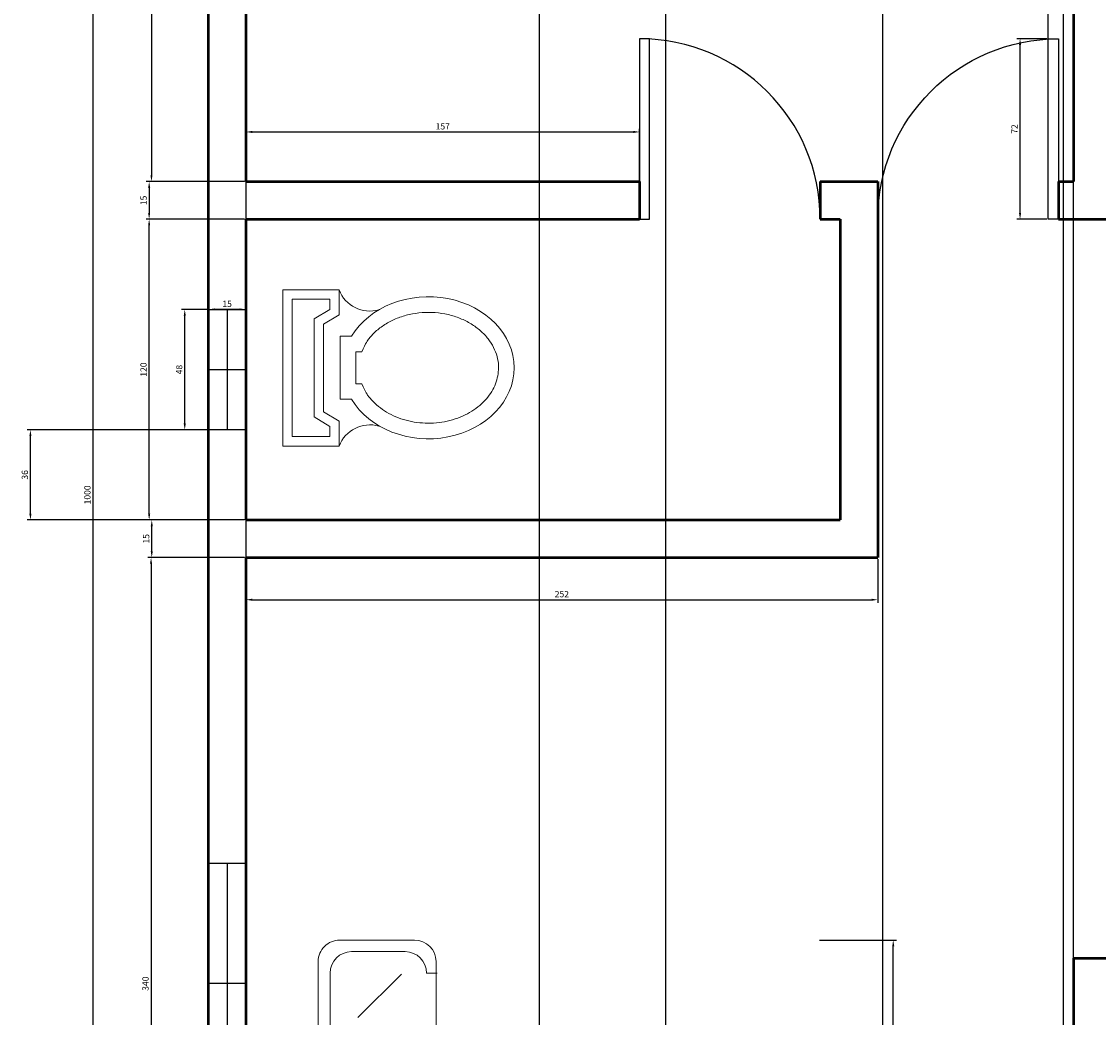
# Model space of a CAD drawing. Units: inches. Extents: x 604 to 3492, y -123 to 1737.
# Tile 7 of 20: x 604 to 1033, y 579 to 977. Entities that reach past the tile are written whole.
import ezdxf

# ---------------------------------------------------------------- set-up
doc = ezdxf.new("R2010")
doc.units = ezdxf.units.IN
for name, color, linetype, lineweight in [('A-ANNO-DIMS', 2, 'Continuous', 18), ('A-DOOR', 3, 'Continuous', 25), ('A-FLOR-FIXT', 9, 'Continuous', 18), ('A-FURN', 8, 'Continuous', 18), ('A-GLAZ', 4, 'Continuous', 25), ('A-WALL', 7, 'Continuous', 50)]:
    doc.layers.add(name, color=color, linetype=linetype, lineweight=lineweight)
doc.styles.get("Standard").update_dxf_attribs({"font": 'arial.ttf'})
doc.dimstyles.new('ISO-25', dxfattribs={"dimtxt": 2.5, "dimasz": 2.5, "dimexe": 1.25, "dimexo": 0.625, "dimtad": 1, "dimtxsty": 'Standard', "dimcen": 2.5, "dimadec": 0, "dimazin": 0, "dimtfac": 1, "dimtmove": 0, "dimatfit": 3, "dimfxl": 1, "dimarcsym": 0})

# ---------------------------------------------------------------- blocks, each defined once
blk = doc.blocks.new('A$C4B324E0D')
for points in [[(-0.4032, -0.0374), (-0.3959, 0.0153), (-0.3883, 0.0678), (-0.3801, 0.1195), (-0.3709, 0.1704), (-0.3605, 0.22), (-0.3485, 0.2679), (-0.3346, 0.314), (-0.3185, 0.3579), (-0.2998, 0.3993), (-0.2783, 0.4378), (-0.2537, 0.4731), (-0.2255, 0.5049), (-0.1936, 0.5331), (-0.1583, 0.5578), (-0.1198, 0.5793), (-0.0785, 0.5979), (-0.0346, 0.614), (0.0115, 0.628), (0.0595, 0.64), (0.1091, 0.6504), (0.1599, 0.6595), (0.2117, 0.6678), (0.2641, 0.6753), (0.3168, 0.6826)], [(0.3768, 0.6826), (0.3168, 0.6826)], [(0.9768, 0.6826), (0.6168, 0.6826)], [(1.5769, 0.6826), (1.2168, 0.6826)], [(1.8168, 0.6826), (2.2368, 0.6826)], [(-0.3432, -0.0374), (-0.3369, 0.0114), (-0.3303, 0.0599), (-0.3232, 0.1078), (-0.3151, 0.1548), (-0.3059, 0.2006), (-0.2951, 0.2449), (-0.2826, 0.2874), (-0.2681, 0.3278), (-0.2511, 0.3658), (-0.2315, 0.4011), (-0.2089, 0.4335), (-0.1831, 0.4625), (-0.1538, 0.488), (-0.1214, 0.5102), (-0.086, 0.5294), (-0.0479, 0.546), (-0.0075, 0.5602), (0.035, 0.5722), (0.0793, 0.5825), (0.125, 0.5914), (0.172, 0.599), (0.2198, 0.6057), (0.2682, 0.6119), (0.3168, 0.6177)], [(0.3168, 0.6177), (0.3168, 0.6177)], [(0.9168, 0.6177), (0.6768, 0.6177)], [(1.5168, 0.6177), (1.2768, 0.6177)], [(2.1704, 0.6177), (1.8704, 0.6177)], [(0.4968, 0.0226), (0.4968, 0.5626)], [(0.4968, 0.5626), (0.4968, 0.0226), (1.0968, 0.0226)], [(1.0968, 0.5626), (1.0968, 0.0226), (1.6968, 0.0226)], [(1.0968, 0.0226), (1.0968, 0.5626)], [(1.6968, 0.0226), (1.6968, 0.5626)], [(2.2368, 0.0226), (1.6968, 0.0226), (1.6968, 0.5626)], [(2.3569, 0.5626), (2.3569, 0.1426)], [(0.4968, 0.4977), (0.4368, 0.4977), (0.4368, 0.4977)], [(0.5569, 0.4977), (0.5569, 0.4977), (0.4968, 0.4977)], [(1.0968, 0.4977), (1.0368, 0.4977), (1.0368, 0.4977)], [(1.1569, 0.4977), (1.1569, 0.4977), (1.0968, 0.4977)], [(1.6969, 0.4977), (1.6368, 0.4977), (1.6368, 0.4977)], [(1.7504, 0.4977), (1.7504, 0.4977), (1.6904, 0.4977)], [(2.2904, 0.1977), (2.2904, 0.4977)], [(0.255, 0.4573), (0.1211, 0.2495)], [(0.9111, 0.4573), (0.6711, 0.2173)], [(1.527, 0.4573), (1.287, 0.2173)], [(2.0759, 0.4573), (1.8359, 0.2173)], [(-0.1199, 0.1664), (0.0943, -0.0414)], [(2.1704, 0.0177), (2.1704, 0.0777), (2.1704, 0.0777)], [(0.4968, 0.0226), (0.3768, 0.0226)], [(-0.4032, -0.0974), (-0.4032, -0.0374)], [(-0.3432, -0.0374), (-0.3432, -0.0374)], [(0.2568, -0.0974), (0.2568, -0.2174)], [(-0.2232, -0.2174), (-0.2232, -0.1574), (-0.2232, -0.1574)], [(-0.2832, -0.8174), (0.2568, -0.8174), (0.2568, -0.2174)], [(0.2568, -0.2174), (-0.2832, -0.2174)], [(0.2568, -0.2174), (-0.2832, -0.2174)], [(-0.2183, -0.2174), (-0.2183, -0.2774), (-0.2183, -0.2774)], [(-0.4032, -0.3374), (-0.4032, -0.6974)], [(-0.3383, -0.3974), (-0.3383, -0.6374)], [(-0.2136, -0.3946), (0.0264, -0.6346)], [(-0.2183, -0.7574), (-0.2183, -0.7574), (-0.2183, -0.8174)], [(0.2568, -0.8174), (-0.2832, -0.8174)], [(-0.2732, -0.8174), (0.2568, -0.8174), (0.2568, -1.3475)], [(-0.208, -0.8126), (-0.208, -0.8715), (-0.208, -0.8715)], [(0.2568, -0.8174), (0.2568, -1.3475)], [(-0.391, -1.3475), (-0.391, -0.9352)], [(-0.3258, -0.9893), (-0.3258, -1.2838)], [(-0.1734, -1.0387), (0.0666, -1.2787)], [(0.2043, -1.2838), (0.2043, -1.2838), (0.2632, -1.2838)], [(-0.208, -1.4016), (0.0865, -1.4016)], [(0.1391, -1.4653), (-0.2732, -1.4653)]]:
    blk.add_lwpolyline(points)
for centre, radius, start, end in [((0.3768, 0.5626), 0.12, 0, 90), ((0.6168, 0.5626), 0.12, 90, 180), ((0.9768, 0.5626), 0.12, 0, 90), ((1.2168, 0.5626), 0.12, 90, 180), ((1.5769, 0.5626), 0.12, 0, 90), ((1.8168, 0.5626), 0.12, 90, 180), ((2.2368, 0.5626), 0.12, 0, 90), ((0.3168, 0.4977), 0.12, 0, 90), ((0.6768, 0.4977), 0.12, 90, 180), ((0.9168, 0.4977), 0.12, 0, 90), ((1.2768, 0.4977), 0.12, 90, 180), ((1.5168, 0.4977), 0.12, 0, 90), ((1.8704, 0.4977), 0.12, 90, 180), ((2.1704, 0.4977), 0.12, 0, 90), ((2.1704, 0.1977), 0.12, 270, 0), ((2.2368, 0.1426), 0.12, 270, 0), ((0.3768, -0.0974), 0.12, 90, 180), ((-0.2232, -0.0374), 0.12, 180, 270), ((-0.2832, -0.0974), 0.12, 179.9997, 270), ((-0.2832, -0.3374), 0.12, 90, 180), ((-0.2183, -0.3974), 0.12, 90, 180), ((-0.2183, -0.6374), 0.12, 180, 270), ((-0.2832, -0.6974), 0.12, 179.9997, 270), ((-0.2732, -0.9352), 0.1178, 90, 180), ((-0.208, -0.9893), 0.1178, 90, 180), ((-0.208, -1.2838), 0.1178, 180, 270), ((0.0865, -1.2838), 0.1178, 270, 0), ((-0.2732, -1.3475), 0.1178, 179.9997, 270), ((0.1391, -1.3475), 0.1178, 270, 0)]:
    blk.add_arc(centre, radius, start, end)
blk = doc.blocks.new('A$C58C6152E')
at = {"xscale": 1.5, "yscale": 1.5, "zscale": 1.5, "rotation": 90}
blk.add_blockref('A$C4B324E0D', (1.0239, 0.6047), dxfattribs=at)
blk = doc.blocks.new('A$C15DC316E')
at = {"xscale": -1, "rotation": 270}
blk.add_blockref('A$C58C6152E', (0, 0), dxfattribs=at)
blk = doc.blocks.new('A$C7C8779AE')
for p, q in [((0, 0.7405), (0, 0.5605)), ((0.5, 0.7405), (0, 0.7405)), ((0.5, 0.5605), (0.5, 0.7405)), ((0.47, 0.7105), (0.03, 0.7105)), ((0.03, 0.7105), (0.03, 0.5905)), ((0.47, 0.5905), (0.47, 0.7105)), ((0.093, 0.6405), (0.063, 0.5905)), ((0.093, 0.6405), (0.407, 0.6405)), ((0.437, 0.5905), (0.407, 0.6405)), ((0.03, 0.5905), (0.063, 0.5905)), ((0.11, 0.6105), (0.08, 0.5605)), ((0.11, 0.6105), (0.39, 0.6105)), ((0.42, 0.5605), (0.39, 0.6105)), ((0.437, 0.5905), (0.47, 0.5905)), ((0, 0.5605), (0.08, 0.5605)), ((0.1497, 0.557), (0.1497, 0.5203)), ((0.1497, 0.557), (0.3514, 0.557)), ((0.3514, 0.557), (0.3514, 0.5203)), ((0.42, 0.5605), (0.5, 0.5605)), ((0.1997, 0.507), (0.1997, 0.4879)), ((0.1997, 0.507), (0.3014, 0.507)), ((0.3014, 0.507), (0.3014, 0.4879))]:
    blk.add_line(p, q)
for centre, start, end in [((-0.0386, 0.4613), 344.642, 68.7339), ((0.5386, 0.4613), 111.2661, 195.358)]:
    blk.add_arc(centre, 0.1064, start, end)
blk.add_ellipse((0.2506, 0.2744), major_axis=(0, 0.2744), ratio=0.828948, start_param=0.459479, end_param=5.823706)
blk.add_open_spline([(0.1997, 0.4879), (0.1697, 0.474), (0.1642, 0.4702), (0.1512, 0.4602), (0.1438, 0.4535), (0.1298, 0.4388), (0.1233, 0.4306), (0.1111, 0.4131), (0.1055, 0.4037), (0.0956, 0.3838), (0.0912, 0.3733), (0.0838, 0.3516), (0.0808, 0.3403), (0.0762, 0.3172), (0.0746, 0.3055), (0.073, 0.2817), (0.0729, 0.2698), (0.0743, 0.246), (0.0758, 0.2342), (0.0801, 0.2111), (0.0831, 0.1998), (0.0903, 0.1779), (0.0945, 0.1673), (0.1043, 0.1473), (0.1098, 0.1378), (0.1218, 0.12), (0.1283, 0.1118), (0.1421, 0.0968), (0.1494, 0.09), (0.1646, 0.078), (0.1725, 0.0728), (0.1887, 0.064), (0.1969, 0.0603), (0.2137, 0.0547), (0.2222, 0.0527), (0.2392, 0.0502), (0.2478, 0.0498), (0.2664, 0.0505), (0.2764, 0.052), (0.2963, 0.0573), (0.3061, 0.061), (0.3253, 0.0707), (0.3346, 0.0766), (0.3525, 0.0906), (0.3611, 0.0987), (0.3771, 0.1169), (0.3845, 0.127), (0.3978, 0.1488), (0.4037, 0.1605), (0.4137, 0.1853), (0.4178, 0.1983), (0.424, 0.2251), (0.4261, 0.2389), (0.4282, 0.2668), (0.4283, 0.2809), (0.4262, 0.3088), (0.4241, 0.3226), (0.418, 0.3495), (0.414, 0.3625), (0.404, 0.3873), (0.3982, 0.3991), (0.385, 0.421), (0.3776, 0.4311), (0.3617, 0.4494), (0.3531, 0.4575), (0.3382, 0.4693), (0.3321, 0.4736), (0.3014, 0.4879)], degree=3, knots=[0.459479, 0.459479, 0.459479, 0.459479, 0.567422, 0.567422, 0.720865, 0.720865, 0.874307, 0.874307, 1.02775, 1.02775, 1.181192, 1.181192, 1.334635, 1.334635, 1.488077, 1.488077, 1.64152, 1.64152, 1.794963, 1.794963, 1.948405, 1.948405, 2.101848, 2.101848, 2.25529, 2.25529, 2.408733, 2.408733, 2.562175, 2.562175, 2.715618, 2.715618, 2.86906, 2.86906, 3.022503, 3.022503, 3.175946, 3.175946, 3.356457, 3.356457, 3.536968, 3.536968, 3.717479, 3.717479, 3.89799, 3.89799, 4.078501, 4.078501, 4.259012, 4.259012, 4.439523, 4.439523, 4.620035, 4.620035, 4.800546, 4.800546, 4.981057, 4.981057, 5.161568, 5.161568, 5.342079, 5.342079, 5.52259, 5.52259, 5.703101, 5.703101, 5.823706, 5.823706, 5.823706, 5.823706])
blk = doc.blocks.new('*D22')
at = {"layer": 'A-ANNO-DIMS', "color": 0, "lineweight": -2, "transparency": 16777216}
for p, q in [((692.39, 1272.7), (654.09, 1272.7)), ((655.34, 1270.2), (655.34, 915.2)), ((692.39, 912.7), (654.09, 912.7))]:
    blk.add_line(p, q, dxfattribs=at)
at = {"layer": 'A-ANNO-DIMS', "color": 0, "transparency": 16777216}
for points in [[(654.92, 1270.2), (655.75, 1270.2), (655.34, 1272.7)], [(654.92, 915.2), (655.75, 915.2), (655.34, 912.7)]]:
    blk.add_solid(points, dxfattribs=at)
at = {"layer": 'Defpoints', "color": 0, "transparency": 16777216}
for p in [(693.01, 1272.7), (655.34, 912.7), (693.01, 912.7)]:
    blk.add_point(p, dxfattribs=at)
at = {"layer": 'A-ANNO-DIMS', "color": 0, "transparency": 16777216, "insert": (653.44, 1092.7), "char_height": 2.5, "attachment_point": 5, "rotation": 90}
blk.add_mtext('360', dxfattribs=at)
blk = doc.blocks.new('*D23')
at = {"layer": 'A-ANNO-DIMS', "color": 0, "lineweight": -2, "transparency": 16777216}
for p, q in [((692.39, 912.7), (653.16, 912.7)), ((654.41, 910.2), (654.41, 900.2)), ((692.39, 897.7), (653.16, 897.7))]:
    blk.add_line(p, q, dxfattribs=at)
at = {"layer": 'A-ANNO-DIMS', "color": 0, "transparency": 16777216}
for points in [[(654, 910.2), (654.83, 910.2), (654.41, 912.7)], [(654, 900.2), (654.83, 900.2), (654.41, 897.7)]]:
    blk.add_solid(points, dxfattribs=at)
at = {"layer": 'Defpoints', "color": 0, "transparency": 16777216}
for p in [(693.01, 912.7), (654.41, 897.7), (693.01, 897.7)]:
    blk.add_point(p, dxfattribs=at)
at = {"layer": 'A-ANNO-DIMS', "color": 0, "transparency": 16777216, "insert": (652.51, 905.2), "char_height": 2.5, "attachment_point": 5, "rotation": 90}
blk.add_mtext('15', dxfattribs=at)
blk = doc.blocks.new('*D24')
at = {"layer": 'A-ANNO-DIMS', "color": 0, "lineweight": -2, "transparency": 16777216}
for p, q in [((692.39, 897.7), (653.16, 897.7)), ((654.41, 780.2), (654.41, 895.2)), ((692.39, 777.7), (653.16, 777.7))]:
    blk.add_line(p, q, dxfattribs=at)
at = {"layer": 'A-ANNO-DIMS', "color": 0, "transparency": 16777216}
for points in [[(654, 895.2), (654.83, 895.2), (654.41, 897.7)], [(654, 780.2), (654.83, 780.2), (654.41, 777.7)]]:
    blk.add_solid(points, dxfattribs=at)
at = {"layer": 'Defpoints', "color": 0, "transparency": 16777216}
for p in [(654.41, 897.7), (693.01, 897.7), (693.01, 777.7)]:
    blk.add_point(p, dxfattribs=at)
at = {"layer": 'A-ANNO-DIMS', "color": 0, "transparency": 16777216, "insert": (652.51, 837.7), "char_height": 2.5, "attachment_point": 5, "rotation": 90}
blk.add_mtext('120', dxfattribs=at)
blk = doc.blocks.new('*D25')
at = {"layer": 'A-ANNO-DIMS', "color": 0, "lineweight": -2, "transparency": 16777216}
for p, q in [((692.39, 777.7), (654.2, 777.7)), ((655.45, 765.2), (655.45, 775.2)), ((692.39, 762.7), (654.2, 762.7))]:
    blk.add_line(p, q, dxfattribs=at)
at = {"layer": 'A-ANNO-DIMS', "color": 0, "transparency": 16777216}
for points in [[(655.04, 775.2), (655.87, 775.2), (655.45, 777.7)], [(655.04, 765.2), (655.87, 765.2), (655.45, 762.7)]]:
    blk.add_solid(points, dxfattribs=at)
at = {"layer": 'Defpoints', "color": 0, "transparency": 16777216}
for p in [(655.45, 777.7), (693.01, 777.7), (693.01, 762.7)]:
    blk.add_point(p, dxfattribs=at)
at = {"layer": 'A-ANNO-DIMS', "color": 0, "transparency": 16777216, "insert": (653.55, 770.2), "char_height": 2.5, "attachment_point": 5, "rotation": 90}
blk.add_mtext('15', dxfattribs=at)
blk = doc.blocks.new('*D26')
at = {"layer": 'A-ANNO-DIMS', "color": 0, "lineweight": -2, "transparency": 16777216}
for p, q in [((692.39, 762.7), (653.92, 762.7)), ((655.17, 760.2), (655.17, 425.2)), ((692.39, 422.7), (653.92, 422.7))]:
    blk.add_line(p, q, dxfattribs=at)
at = {"layer": 'A-ANNO-DIMS', "color": 0, "transparency": 16777216}
for points in [[(654.75, 760.2), (655.58, 760.2), (655.17, 762.7)], [(654.75, 425.2), (655.58, 425.2), (655.17, 422.7)]]:
    blk.add_solid(points, dxfattribs=at)
at = {"layer": 'Defpoints', "color": 0, "transparency": 16777216}
for p in [(693.01, 762.7), (655.17, 422.7), (693.01, 422.7)]:
    blk.add_point(p, dxfattribs=at)
at = {"layer": 'A-ANNO-DIMS', "color": 0, "transparency": 16777216, "insert": (653.26, 592.7), "char_height": 2.5, "attachment_point": 5, "rotation": 90}
blk.add_mtext('340', dxfattribs=at)
blk = doc.blocks.new('*D30')
at = {"layer": 'A-ANNO-DIMS', "color": 0, "lineweight": -2, "transparency": 16777216}
for p, q in [((693.01, 913.33), (693.01, 933.76)), ((695.51, 932.51), (847.51, 932.51)), ((850.01, 913.33), (850.01, 933.76))]:
    blk.add_line(p, q, dxfattribs=at)
at = {"layer": 'A-ANNO-DIMS', "color": 0, "transparency": 16777216}
for points in [[(695.51, 932.93), (695.51, 932.1), (693.01, 932.51)], [(847.51, 932.93), (847.51, 932.1), (850.01, 932.51)]]:
    blk.add_solid(points, dxfattribs=at)
at = {"layer": 'Defpoints', "color": 0, "transparency": 16777216}
for p in [(850.01, 932.51), (693.01, 912.7), (850.01, 912.7)]:
    blk.add_point(p, dxfattribs=at)
at = {"layer": 'A-ANNO-DIMS', "color": 0, "transparency": 16777216, "insert": (771.51, 934.42), "char_height": 2.5, "attachment_point": 5}
blk.add_mtext('157', dxfattribs=at)
blk = doc.blocks.new('*D31')
at = {"layer": 'A-ANNO-DIMS', "color": 0, "lineweight": -2, "transparency": 16777216}
for p, q in [((693.01, 762.08), (693.01, 744.63)), ((945.01, 762.08), (945.01, 744.63)), ((695.51, 745.88), (942.51, 745.88))]:
    blk.add_line(p, q, dxfattribs=at)
at = {"layer": 'A-ANNO-DIMS', "color": 0, "transparency": 16777216}
for points in [[(695.51, 746.29), (695.51, 745.46), (693.01, 745.88)], [(942.51, 746.29), (942.51, 745.46), (945.01, 745.88)]]:
    blk.add_solid(points, dxfattribs=at)
at = {"layer": 'Defpoints', "color": 0, "transparency": 16777216}
for p in [(693.01, 762.7), (945.01, 762.7), (945.01, 745.88)]:
    blk.add_point(p, dxfattribs=at)
at = {"layer": 'A-ANNO-DIMS', "color": 0, "transparency": 16777216, "insert": (819.01, 747.78), "char_height": 2.5, "attachment_point": 5}
blk.add_mtext('252', dxfattribs=at)
blk = doc.blocks.new('*D32')
at = {"layer": 'A-ANNO-DIMS', "color": 0, "lineweight": -2, "transparency": 16777216}
for p, q in [((1012.39, 969.7), (1000.49, 969.7)), ((1001.74, 900.2), (1001.74, 967.2)), ((1012.39, 897.7), (1000.49, 897.7))]:
    blk.add_line(p, q, dxfattribs=at)
at = {"layer": 'A-ANNO-DIMS', "color": 0, "transparency": 16777216}
for points in [[(1001.32, 967.2), (1002.16, 967.2), (1001.74, 969.7)], [(1001.32, 900.2), (1002.16, 900.2), (1001.74, 897.7)]]:
    blk.add_solid(points, dxfattribs=at)
at = {"layer": 'Defpoints', "color": 0, "transparency": 16777216}
for p in [(1001.74, 969.7), (1013.01, 969.7), (1013.01, 897.7)]:
    blk.add_point(p, dxfattribs=at)
at = {"layer": 'A-ANNO-DIMS', "color": 0, "transparency": 16777216, "insert": (999.86, 933.7), "char_height": 2.5, "attachment_point": 5, "rotation": 90}
blk.add_mtext('72', dxfattribs=at)
blk = doc.blocks.new('*D35')
at = {"layer": 'A-ANNO-DIMS', "color": 0, "lineweight": -2, "transparency": 16777216}
for p, q in [((678.01, 814.33), (678.01, 862.95)), ((690.51, 861.7), (680.51, 861.7)), ((693.01, 814.33), (693.01, 862.95))]:
    blk.add_line(p, q, dxfattribs=at)
at = {"layer": 'A-ANNO-DIMS', "color": 0, "transparency": 16777216}
for points in [[(680.51, 862.12), (680.51, 861.28), (678.01, 861.7)], [(690.51, 862.12), (690.51, 861.28), (693.01, 861.7)]]:
    blk.add_solid(points, dxfattribs=at)
at = {"layer": 'Defpoints', "color": 0, "transparency": 16777216}
for p in [(678.01, 861.7), (678.01, 813.7), (693.01, 813.7)]:
    blk.add_point(p, dxfattribs=at)
at = {"layer": 'A-ANNO-DIMS', "color": 0, "transparency": 16777216, "insert": (685.51, 863.6), "char_height": 2.5, "attachment_point": 5}
blk.add_mtext('15', dxfattribs=at)
blk = doc.blocks.new('*D36')
at = {"layer": 'A-ANNO-DIMS', "color": 0, "lineweight": -2, "transparency": 16777216}
for p, q in [((677.39, 861.7), (667.36, 861.7)), ((668.61, 816.2), (668.61, 859.2)), ((677.39, 813.7), (667.36, 813.7))]:
    blk.add_line(p, q, dxfattribs=at)
at = {"layer": 'A-ANNO-DIMS', "color": 0, "transparency": 16777216}
for points in [[(668.19, 859.2), (669.03, 859.2), (668.61, 861.7)], [(668.19, 816.2), (669.03, 816.2), (668.61, 813.7)]]:
    blk.add_solid(points, dxfattribs=at)
at = {"layer": 'Defpoints', "color": 0, "transparency": 16777216}
for p in [(668.61, 861.7), (678.01, 861.7), (678.01, 813.7)]:
    blk.add_point(p, dxfattribs=at)
at = {"layer": 'A-ANNO-DIMS', "color": 0, "transparency": 16777216, "insert": (666.71, 837.7), "char_height": 2.5, "attachment_point": 5, "rotation": 90}
blk.add_mtext('48', dxfattribs=at)
blk = doc.blocks.new('*D37')
at = {"layer": 'A-ANNO-DIMS', "color": 0, "lineweight": -2, "transparency": 16777216}
for p, q in [((677.39, 1287.7), (630.76, 1287.7)), ((632.01, 1285.2), (632.01, 290.2)), ((677.39, 287.7), (630.76, 287.7))]:
    blk.add_line(p, q, dxfattribs=at)
at = {"layer": 'A-ANNO-DIMS', "color": 0, "transparency": 16777216}
for points in [[(631.59, 1285.2), (632.42, 1285.2), (632.01, 1287.7)], [(631.59, 290.2), (632.42, 290.2), (632.01, 287.7)]]:
    blk.add_solid(points, dxfattribs=at)
at = {"layer": 'Defpoints', "color": 0, "transparency": 16777216}
for p in [(678.01, 1287.7), (632.01, 287.7), (678.01, 287.7)]:
    blk.add_point(p, dxfattribs=at)
at = {"layer": 'A-ANNO-DIMS', "color": 0, "transparency": 16777216, "insert": (630.1, 787.7), "char_height": 2.5, "attachment_point": 5, "rotation": 90}
blk.add_mtext('1000', dxfattribs=at)
blk = doc.blocks.new('DOOR-SWING-72')
for p, q in [((0, 72), (0, 0)), ((0, 0), (4, 0)), ((0, 0), (4, 0))]:
    blk.add_line(p, q)
blk.add_lwpolyline([(0, 72), (0, 0), (4, 0), (4, 72)], close=True)
blk.add_arc((0, 0), 72, 0, 90)
blk = doc.blocks.new('WIN-96')
for p, q in [((15, 96), (0, 96)), ((7.5, 96), (7.5, 0)), ((15, 96), (15, 0)), ((15, 48), (0, 48))]:
    blk.add_line(p, q)
blk.add_lwpolyline([(0, 96), (0, 0), (15, 0), (15, 96)], close=True)
blk = doc.blocks.new('WIN-48')
for p, q in [((0, 48), (15, 48)), ((7.5, 48), (7.5, 0)), ((15, 48), (15, 0)), ((0, 24), (15, 24))]:
    blk.add_line(p, q)
blk.add_lwpolyline([(15, 0), (0, 0), (0, 48), (15, 48)], close=True)
blk = doc.blocks.new('*D80')
at = {"layer": 'A-ANNO-DIMS', "color": 0, "lineweight": -2, "transparency": 16777216}
for p, q in [((921.76, 610.08), (952.41, 610.08)), ((951.16, 456.8), (951.16, 607.58)), ((921.76, 454.3), (952.41, 454.3))]:
    blk.add_line(p, q, dxfattribs=at)
at = {"layer": 'A-ANNO-DIMS', "color": 0, "transparency": 16777216}
for points in [[(950.75, 607.58), (951.58, 607.58), (951.16, 610.08)], [(950.75, 456.8), (951.58, 456.8), (951.16, 454.3)]]:
    blk.add_solid(points, dxfattribs=at)
at = {"layer": 'Defpoints', "color": 0, "transparency": 16777216}
for p in [(921.14, 610.08), (951.16, 610.08), (921.14, 454.3)]:
    blk.add_point(p, dxfattribs=at)
at = {"layer": 'A-ANNO-DIMS', "color": 0, "transparency": 16777216, "insert": (949.26, 532.19), "char_height": 2.5, "attachment_point": 5, "rotation": 90}
blk.add_mtext('156', dxfattribs=at)
blk = doc.blocks.new('*D85')
at = {"layer": 'A-ANNO-DIMS', "color": 0, "lineweight": -2, "transparency": 16777216}
for p, q in [((693.01, 1272.08), (693.01, 67.77)), ((810.01, 1272.08), (810.01, 67.77)), ((695.51, 69.02), (807.51, 69.02))]:
    blk.add_line(p, q, dxfattribs=at)
at = {"layer": 'A-ANNO-DIMS', "color": 0, "transparency": 16777216}
for points in [[(695.51, 69.44), (695.51, 68.61), (693.01, 69.02)], [(807.51, 69.44), (807.51, 68.61), (810.01, 69.02)]]:
    blk.add_solid(points, dxfattribs=at)
at = {"layer": 'Defpoints', "color": 0, "transparency": 16777216}
for p in [(693.01, 1272.7), (810.01, 1272.7), (810.01, 69.02)]:
    blk.add_point(p, dxfattribs=at)
at = {"layer": 'A-ANNO-DIMS', "color": 0, "transparency": 16777216, "insert": (751.51, 70.9), "char_height": 2.5, "attachment_point": 5}
blk.add_mtext('117', dxfattribs=at)
blk = doc.blocks.new('*D90')
at = {"layer": 'A-ANNO-DIMS', "color": 0, "lineweight": -2, "transparency": 16777216}
for p, q in [((1016.51, 1358.65), (1014.01, 1358.65)), ((1019.01, 423.33), (1019.01, 1359.9)), ((1023.01, 1358.65), (1019.01, 1358.65)), ((1023.01, 423.33), (1023.01, 1359.9)), ((1025.51, 1358.65), (1028.01, 1358.65))]:
    blk.add_line(p, q, dxfattribs=at)
at = {"layer": 'A-ANNO-DIMS', "color": 0, "transparency": 16777216}
for points in [[(1016.51, 1359.07), (1016.51, 1358.23), (1019.01, 1358.65)], [(1025.51, 1359.07), (1025.51, 1358.23), (1023.01, 1358.65)]]:
    blk.add_solid(points, dxfattribs=at)
at = {"layer": 'Defpoints', "color": 0, "transparency": 16777216}
for p in [(1019.01, 1358.65), (1019.01, 422.7), (1023.01, 422.7)]:
    blk.add_point(p, dxfattribs=at)
at = {"layer": 'A-ANNO-DIMS', "color": 0, "transparency": 16777216, "insert": (1021.01, 1360.53), "char_height": 2.5, "attachment_point": 5}
blk.add_mtext('4', dxfattribs=at)
blk = doc.blocks.new('*D91')
at = {"layer": 'A-ANNO-DIMS', "color": 0, "lineweight": -2, "transparency": 16777216}
for p, q in [((860.51, 408.33), (860.51, 1359.9)), ((863.01, 1358.65), (944.51, 1358.65)), ((947.01, 408.33), (947.01, 1359.9))]:
    blk.add_line(p, q, dxfattribs=at)
at = {"layer": 'A-ANNO-DIMS', "color": 0, "transparency": 16777216}
for points in [[(863.01, 1359.07), (863.01, 1358.23), (860.51, 1358.65)], [(944.51, 1359.07), (944.51, 1358.23), (947.01, 1358.65)]]:
    blk.add_solid(points, dxfattribs=at)
at = {"layer": 'Defpoints', "color": 0, "transparency": 16777216}
for p in [(947.01, 1358.65), (860.51, 407.7), (947.01, 407.7)]:
    blk.add_point(p, dxfattribs=at)
at = {"layer": 'A-ANNO-DIMS', "color": 0, "transparency": 16777216, "insert": (903.76, 1360.55), "char_height": 2.5, "attachment_point": 5}
blk.add_mtext('86.5', dxfattribs=at)
blk = doc.blocks.new('*D92')
at = {"layer": 'A-ANNO-DIMS', "color": 0, "lineweight": -2, "transparency": 16777216}
for p, q in [((677.39, 813.7), (605.81, 813.7)), ((607.06, 780.2), (607.06, 811.2)), ((692.39, 777.7), (605.81, 777.7))]:
    blk.add_line(p, q, dxfattribs=at)
at = {"layer": 'A-ANNO-DIMS', "color": 0, "transparency": 16777216}
for points in [[(606.64, 811.2), (607.48, 811.2), (607.06, 813.7)], [(606.64, 780.2), (607.48, 780.2), (607.06, 777.7)]]:
    blk.add_solid(points, dxfattribs=at)
at = {"layer": 'Defpoints', "color": 0, "transparency": 16777216}
for p in [(607.06, 813.7), (678.01, 813.7), (693.01, 777.7)]:
    blk.add_point(p, dxfattribs=at)
at = {"layer": 'A-ANNO-DIMS', "color": 0, "transparency": 16777216, "insert": (605.16, 795.7), "char_height": 2.5, "attachment_point": 5, "rotation": 90}
blk.add_mtext('36', dxfattribs=at)
blk = doc.blocks.new('*D99')
at = {"layer": 'A-ANNO-DIMS', "color": 0, "lineweight": -2, "transparency": 16777216}
for p, q in [((1013.01, 898.33), (1013.01, 1359.9)), ((1015.51, 1358.65), (1020.51, 1358.65)), ((1023.01, 913.33), (1023.01, 1359.9))]:
    blk.add_line(p, q, dxfattribs=at)
at = {"layer": 'A-ANNO-DIMS', "color": 0, "transparency": 16777216}
for points in [[(1015.51, 1359.07), (1015.51, 1358.23), (1013.01, 1358.65)], [(1020.51, 1359.07), (1020.51, 1358.23), (1023.01, 1358.65)]]:
    blk.add_solid(points, dxfattribs=at)
at = {"layer": 'Defpoints', "color": 0, "transparency": 16777216}
for p in [(1023.01, 1358.65), (1023.01, 912.7), (1013.01, 897.7)]:
    blk.add_point(p, dxfattribs=at)
at = {"layer": 'A-ANNO-DIMS', "color": 0, "transparency": 16777216, "insert": (1018.01, 1360.55), "char_height": 2.5, "attachment_point": 5}
blk.add_mtext('10', dxfattribs=at)

msp = doc.modelspace()

# ---------------------------------------------------------------- linework, layer by layer
at = {"layer": 'A-WALL'}
for p, q in [((678.0111, 1287.7004), (678.0111, 287.7004)), ((693.0111, 1272.7004), (693.0111, 912.7004)), ((1023.0111, 1272.7004), (1023.0111, 912.7004)), ((693.0111, 912.7004), (850.0111, 912.7004)), ((850.0111, 912.7004), (850.0111, 897.7004)), ((922.0111, 912.7004), (922.0111, 897.7004)), ((922.0111, 912.7004), (945.0111, 912.7004)), ((945.0111, 912.7004), (945.0111, 897.7004)), ((1017.0111, 912.7004), (1017.0111, 897.7004)), ((1017.0111, 912.7004), (1023.0111, 912.7004)), ((678.0111, 897.7004), (678.0111, 777.7004)), ((693.0111, 897.7004), (850.0111, 897.7004)), ((693.0111, 897.7004), (693.0111, 777.7004)), ((922.0111, 897.7004), (930.0111, 897.7004)), ((930.0111, 897.7004), (930.0111, 777.7004)), ((945.0111, 897.7004), (945.0111, 777.7004)), ((1017.0111, 897.7004), (1038.0111, 897.7004)), ((693.0111, 777.7004), (930.0111, 777.7004)), ((945.0111, 777.7004), (945.0111, 762.7004)), ((693.0111, 762.7004), (945.0111, 762.7004)), ((693.0111, 762.7004), (693.0111, 422.7004)), ((693.0111, 762.7004), (693.0111, 422.7004))]:
    msp.add_line(p, q, dxfattribs=at)
msp.add_lwpolyline([(1038.0111, 602.7004), (1023.0111, 602.7004), (1023.0111, 422.7004)], dxfattribs=at)

# ---------------------------------------------------------------- block references
at = {"layer": 'A-DOOR'}
msp.add_blockref('DOOR-SWING-72', (850.0111, 897.7004), dxfattribs=at)
at = {"layer": 'A-DOOR', "extrusion": (0, 0, -1), "zscale": -1}
msp.add_blockref('DOOR-SWING-72', (-1017.0111, 897.7004), dxfattribs=at)
at = {"layer": 'A-FLOR-FIXT', "xscale": 124.5715386448482, "yscale": 124.5715386448482, "zscale": 124.5715386448482, "rotation": 90}
msp.add_blockref('A$C7C8779AE', (799.9828, 807.2037), dxfattribs=at)
at = {"layer": 'A-FURN', "xscale": 48.35233930155243, "yscale": 48.35233930155243, "zscale": 48.35233930155243}
msp.add_blockref('A$C15DC316E', (720.9565, 454.2997), dxfattribs=at)
at = {"layer": 'A-GLAZ'}
for name, p in [('WIN-48', (678.0111, 813.7004)), ('WIN-96', (678.0111, 544.7004))]:
    msp.add_blockref(name, p, dxfattribs=at)

# ---------------------------------------------------------------- dimensions: what is measured, and where the dimension line sits
at = {"layer": 'A-ANNO-DIMS'}
for base, p1, p2, override, picture, middle in [((947.0111, 1358.6504), (860.5111, 407.7004), (947.0111, 407.7004), {"dimdec": 1, "dimlfac": 1, "dimrnd": 0, "dimzin": 0, "dimdsep": 46, "dimlunit": 2}, '*D91', (903.7611, 1360.5519)), ((1023.0111, 1358.6504), (1013.0111, 897.7004), (1023.0111, 912.7004), {"dimdec": 0, "dimlfac": 1, "dimrnd": 0, "dimzin": 0, "dimdsep": 46, "dimlunit": 2}, '*D99', (1018.0111, 1360.5519)), ((1019.0111, 1358.6504), (1023.0111, 422.7004), (1019.0111, 422.7004), {"dimdec": 0, "dimlfac": 1, "dimrnd": 0, "dimzin": 0, "dimdsep": 46, "dimlunit": 2}, '*D90', (1021.0111, 1360.5254)), ((810.0111, 69.0242), (693.0111, 1272.7004), (810.0111, 1272.7004), {"dimdec": 0, "dimlfac": 1, "dimrnd": 0, "dimzin": 0, "dimdsep": 46, "dimlunit": 2}, '*D85', (751.5111, 70.9043)), ((850.0111, 932.5141), (693.0111, 912.7004), (850.0111, 912.7004), {"dimclrd": 0, "dimclre": 0, "dimclrt": 0}, '*D30', (771.5111, 934.4156)), ((678.0111, 861.7004), (693.0111, 813.7004), (678.0111, 813.7004), {"dimclrd": 0, "dimclre": 0, "dimclrt": 0}, '*D35', (685.5111, 863.6019)), ((945.0111, 745.8766), (693.0111, 762.7004), (945.0111, 762.7004), {"dimclrd": 0, "dimclre": 0, "dimclrt": 0}, '*D31', (819.0111, 747.7781))]:
    dim = msp.add_linear_dim(base=base, p1=p1, p2=p2, dimstyle='ISO-25', override=override, dxfattribs=at)
    dim.commit()
    dim.dimension.update_dxf_attribs({"geometry": picture, "text_midpoint": middle})
for base, p1, p2, override, picture, middle in [((632.0054, 287.7004), (678.0111, 1287.7004), (678.0111, 287.7004), {"dimclrd": 0, "dimclre": 0, "dimclrt": 0}, '*D37', (630.104, 787.7004)), ((655.3379, 912.7004), (693.0111, 1272.7004), (693.0111, 912.7004), {"dimclrd": 0, "dimclre": 0, "dimclrt": 0}, '*D22', (653.4356, 1092.7004)), ((1001.7395, 969.7004), (1013.0111, 897.7004), (1013.0111, 969.7004), {"dimclrd": 0, "dimclre": 0, "dimclrt": 0}, '*D32', (999.8594, 933.7004)), ((654.4125, 897.7004), (693.0111, 912.7004), (693.0111, 897.7004), {"dimclrd": 0, "dimclre": 0, "dimclrt": 0}, '*D23', (652.5111, 905.2004)), ((654.4125, 897.7004), (693.0111, 777.7004), (693.0111, 897.7004), {"dimclrd": 0, "dimclre": 0, "dimclrt": 0}, '*D24', (652.5111, 837.7004)), ((668.611, 861.7004), (678.0111, 813.7004), (678.0111, 861.7004), {"dimclrd": 0, "dimclre": 0, "dimclrt": 0}, '*D36', (666.7095, 837.7004)), ((607.0611, 813.7004), (693.0111, 777.7004), (678.0111, 813.7004), {"dimdec": 0, "dimlfac": 1, "dimrnd": 0, "dimzin": 0, "dimdsep": 46, "dimlunit": 2}, '*D92', (605.1588, 795.7004)), ((655.4525, 777.7004), (693.0111, 762.7004), (693.0111, 777.7004), {"dimclrd": 0, "dimclre": 0, "dimclrt": 0}, '*D25', (653.551, 770.2004)), ((655.1671, 422.7004), (693.0111, 762.7004), (693.0111, 422.7004), {"dimclrd": 0, "dimclre": 0, "dimclrt": 0}, '*D26', (653.2648, 592.7004)), ((951.1628, 610.0802), (921.1359, 454.2997), (921.1359, 610.0802), {"dimdec": 0, "dimlfac": 1, "dimrnd": 0, "dimzin": 0, "dimdsep": 46, "dimlunit": 2}, '*D80', (949.2614, 532.1899))]:
    dim = msp.add_linear_dim(base=base, p1=p1, p2=p2, angle=90, dimstyle='ISO-25', override=override, dxfattribs=at)
    dim.commit()
    dim.dimension.update_dxf_attribs({"geometry": picture, "text_midpoint": middle})

doc.saveas('drawing.dxf')
